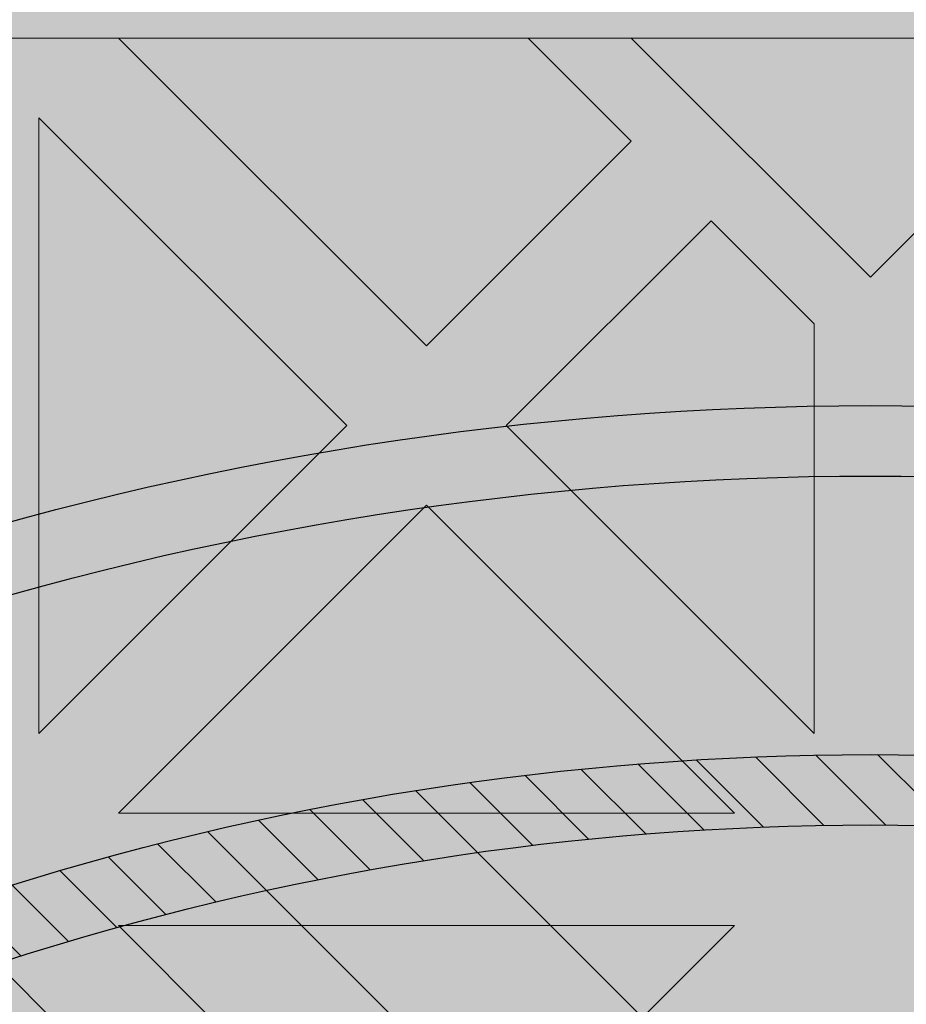
# Model space of a CAD drawing. Units: inches. Extents: x 844 to 2234, y 346 to 1084.
# Tile 81 of 93: x 2001.933 to 2003.94, y 708.742 to 710.971. Entities that reach past the tile are written whole.
import ezdxf

# ---------------------------------------------------------------- set-up
doc = ezdxf.new("R2010")
doc.units = ezdxf.units.IN
doc.header["$MEASUREMENT"] = 0
for name, color, linetype, lineweight in [('A-ANNO-DIMS', 2, 'Continuous', 18), ('furniture', 8, 'Continuous', 18), ('RA-AP-01$0$INT', 35, 'Continuous', 5)]:
    doc.layers.add(name, color=color, linetype=linetype, lineweight=lineweight)
doc.layers.add('RA-AP-01$0$FURN', color=3, linetype='Continuous')
doc.layers.add('RA-AP-01$0$WOOD', color=64, linetype='Continuous')
doc.styles.get("Standard").update_dxf_attribs({"font": 'arial.ttf'})
doc.dimstyles.get("Standard").update_dxf_attribs({"dimtxt": 6, "dimasz": 3, "dimexe": 0.18, "dimexo": 0.0625, "dimgap": 0.09, "dimtad": 0, "dimtih": 1, "dimtoh": 1, "dimdec": 1, "dimzin": 0, "dimdsep": 46, "dimlunit": 3, "dimtxsty": 'Standard', "dimblk": 'ARCHTICK', "dimcen": 0.09, "dimadec": 0, "dimazin": 0, "dimtfac": 1, "dimtdec": 1, "dimtofl": 0, "dimtmove": 0, "dimatfit": 3, "dimfxl": 1, "dimtolj": 1, "dimtzin": 0, "dimarcsym": 0})

# ---------------------------------------------------------------- blocks, each defined once
blk = doc.blocks.new('A$C18D01794')
at = {"layer": 'RA-AP-01$0$INT'}
blk.add_hatch(color=256, dxfattribs=at).paths.add_polyline_path([(4.505206456958071, -7.906712009588039), (5.305206456958072, -7.906712009588039), (5.305206456958072, -7.106712009588038), (5.255206456951893, -7.106712009588036), (5.25520645694868, -7.856712009570104), (4.555206456959269, -7.856712009588616), (4.555206456956052, -7.106712009588038), (4.505206456958073, -7.106712009588038)])
h = blk.add_hatch(color=256, dxfattribs=at)
h.paths.add_polyline_path([(4.585917135068448, -7.856712009587804), (4.614201406330596, -7.856712009587056), (4.668846067270487, -7.802067348644738), (4.723490728212344, -7.856712009584164), (4.771774999457151, -7.856712009582887), (4.826419660396886, -7.80206734864072), (4.862780050090322, -7.838427738332541), (4.844495778842715, -7.856712009580965), (4.862780050090411, -7.856712009580482), (4.905206456960182, -7.814285602707865), (4.947632863832445, -7.856712009578238), (4.965917135079675, -7.856712009577755), (4.947632863831759, -7.838427738330656), (4.983993253523576, -7.802067348637219), (5.038637914464627, -7.856712009575829), (5.08692218571208, -7.856712009574554), (5.141566846649976, -7.802067348634224), (5.196211507589851, -7.856712009571666), (5.224495778822615, -7.856712009570916), (4.905206456953975, -7.537422687702283)])
h.paths.add_polyline_path([(4.895206456956031, -7.575706958950402), (4.895206456958921, -7.684996280828174), (4.840561796018589, -7.630351619890275)], flags=16)
h.paths.add_polyline_path([(4.915206456955638, -7.575706958949956), (4.969851117895509, -7.630351619887399), (4.915206456957609, -7.684996280827732)], flags=16)
h.paths.add_polyline_path([(4.826419660395175, -7.644493755514321), (4.881064321335613, -7.699138416452331), (4.771774999456703, -7.69913841645522)], flags=16)
h.paths.add_polyline_path([(4.983993253519558, -7.644493755510815), (5.038637914460456, -7.699138416449285), (4.929348592581548, -7.69913841645126)], flags=16)
h.paths.add_polyline_path([(4.881064321336025, -7.719138416452334), (4.826419660397532, -7.773783077393256), (4.771774999457062, -7.719138416455217)], flags=16)
h.paths.add_polyline_path([(4.929348592582019, -7.71913841645126), (5.038637914460982, -7.719138416449284), (4.983993253522945, -7.773783077389749)], flags=16)
h.paths.add_polyline_path([(4.895206456960191, -7.733280552075633), (4.895206456962115, -7.806001331460164), (4.876922185715016, -7.824285602708492), (4.840561796021581, -7.787925213016675)], flags=16)
h.paths.add_polyline_path([(4.915206456958487, -7.733280552075187), (4.969851117899527, -7.787925213013798), (4.933490728206909, -7.824285602708034), (4.9152064569598, -7.806001331461736)], flags=16)
h.paths.add_polyline_path([(4.757632863832376, -7.733280552079264), (4.812277524772842, -7.787925213017304), (4.757632863834348, -7.842569873958233)], flags=16)
h.paths.add_polyline_path([(4.737632863832376, -7.73328055207979), (4.737632863834348, -7.842569873958701), (4.682988202893906, -7.787925213020692)], flags=16)
h.paths.add_polyline_path([(5.05278005008503, -7.733280552072701), (5.052780050087917, -7.842569873951664), (4.998135389146995, -7.787925213013169)], flags=16)
h.paths.add_polyline_path([(5.072780050085024, -7.733280552072333), (5.127424711025931, -7.787925213010806), (5.072780050087916, -7.842569873951244)], flags=16)
h.paths.add_polyline_path([(4.935917135072783, -7.506712009583784), (5.255206456948811, -7.826001331459767), (5.255206456948932, -7.797717060211899), (5.200561796010279, -7.743072399273238), (5.255206456949403, -7.688427738334128), (5.25520645694961, -7.640143467086677), (5.200561796009787, -7.585498806146837), (5.236922185702417, -7.549138416454212), (5.255206456949919, -7.56742268770172), (5.255206456949998, -7.549138416454178), (5.212780050078687, -7.506712009583814), (5.25520645695036, -7.464285602712145), (5.255206456950438, -7.446001331464763), (5.236922185702424, -7.464285602712779), (5.200561796009796, -7.427925213020149), (5.255206456950753, -7.373280552079203), (5.25520645695096, -7.324996280834394), (5.200561796010322, -7.270351619893748), (5.255206456951428, -7.215706958952649), (5.255206456951547, -7.187422687705071)])
h.paths.add_polyline_path([(5.042988202883395, -7.42792521302065), (5.097632863823085, -7.373280552080975), (5.097632863822622, -7.482569873959883)], flags=16)
h.paths.add_polyline_path([(5.028846067259663, -7.442067348644384), (5.083490728198774, -7.496712009583504), (4.974201406321001, -7.496712009583035)], flags=16)
h.paths.add_polyline_path([(5.117632863823087, -7.37328055208089), (5.172277524762331, -7.42792521302015), (5.11763286382262, -7.482569873959851)], flags=16)
h.paths.add_polyline_path([(5.08349072819877, -7.516712009582191), (5.028846067259652, -7.571356670521302), (4.974201406320998, -7.516712009582638)], flags=16)
h.paths.add_polyline_path([(5.131774999446817, -7.35913841645716), (5.186419660386065, -7.413783077396415), (5.241064321325782, -7.359138416456712)], flags=17)
h.paths.add_polyline_path([(5.131774999446228, -7.496712009583703), (5.186419660386065, -7.442067348643883), (5.222780050079488, -7.478427738337313), (5.204495778832781, -7.496712009584014)], flags=16)
h.paths.add_polyline_path([(5.097632863822613, -7.530854145205813), (5.097632863823061, -7.640143467084723), (5.042988202883383, -7.585498806145032)], flags=16)
h.paths.add_polyline_path([(5.131774999446899, -7.339138416457162), (5.241064321325809, -7.339138416456712), (5.186419660386591, -7.284493755517479)], flags=17)
h.paths.add_polyline_path([(5.131774999446226, -7.516712009581999), (5.204495778830767, -7.516712009581702), (5.22278005007868, -7.534996280829206), (5.186419660386049, -7.571356670521828)], flags=16)
h.paths.add_polyline_path([(5.11763286382262, -7.530854145205852), (5.17227752476232, -7.585498806145562), (5.117632863823064, -7.64014346708481)], flags=16)
h.paths.add_polyline_path([(5.186419660386069, -7.599640941770585), (5.241064321325754, -7.654285602710281), (5.131774999446791, -7.654285602709814)], flags=16)
h.paths.add_polyline_path([(5.131774999446872, -7.674285602709813), (5.24106432132578, -7.674285602710282), (5.186419660386554, -7.728930263649504)], flags=16)
h.paths.add_polyline_path([(5.255206456951811, -7.126001331467467), (5.255206456951895, -7.106712009588038), (4.555206456956052, -7.106712009588038), (4.555206456956136, -7.12600133146746), (4.905206456953973, -7.476001331465289)])
h.paths.add_polyline_path([(4.983993253513404, -7.368930263651977), (4.92934859257295, -7.314285602713969), (5.03863791445186, -7.314285602711063)], flags=16)
h.paths.add_polyline_path([(4.969851117889988, -7.383072399276016), (4.915206456952556, -7.437717060215906), (4.915206456949648, -7.328427738338133)], flags=16)
h.paths.add_polyline_path([(4.929348592572535, -7.294285602713971), (4.983993253511019, -7.239640941773039), (5.038637914451496, -7.294285602711065)], flags=16)
h.paths.add_polyline_path([(5.052780050074912, -7.280143467087016), (4.998135389134438, -7.225498806148989), (5.052780050072919, -7.170854145208052)], flags=16)
h.paths.add_polyline_path([(5.07278005007491, -7.280143467086489), (5.072780050072918, -7.170854145207579), (5.127424711013374, -7.225498806145578)], flags=16)
h.paths.add_polyline_path([(4.89520645695295, -7.437717060216355), (4.840561796013067, -7.383072399278919), (4.895206456950961, -7.328427738338582)], flags=16)
h.paths.add_polyline_path([(4.915206456948365, -7.280143467090674), (4.915206456946434, -7.207422687704125), (4.933490728192729, -7.18913841645701), (4.969851117886972, -7.225498806149623)], flags=16)
h.paths.add_polyline_path([(4.881064321327021, -7.314285602715054), (4.82641966038902, -7.368930263655506), (4.771774999448108, -7.314285602717047)], flags=16)
h.paths.add_polyline_path([(4.895206456950073, -7.280143467091125), (4.840561796009022, -7.225498806152518), (4.876922185700835, -7.18913841645908), (4.895206456948749, -7.207422687706589)], flags=16)
h.paths.add_polyline_path([(4.983993253510392, -7.211356670525576), (4.947632863816944, -7.174996280833758), (4.965917135064043, -7.156712009585847), (5.038637914448995, -7.156712009584522)], flags=16)
h.paths.add_polyline_path([(4.881064321326543, -7.294285602715056), (4.771774999447578, -7.294285602717046), (4.826419660385607, -7.239640941776569)], flags=16)
h.paths.add_polyline_path([(4.905206456946447, -7.19913841645844), (4.862780050074785, -7.156712009587725), (4.947632863816685, -7.156712009586302)], flags=16)
h.paths.add_polyline_path([(5.14156684663679, -7.211356670521528), (5.086922185696452, -7.156712009583639), (5.196211507574223, -7.156712009581651)], flags=16)
h.paths.add_polyline_path([(4.8264196603837, -7.211356670529104), (4.771774999442643, -7.156712009590501), (4.8444957788276, -7.156712009588568), (4.862780050075511, -7.17499628083566)], flags=16)
h.paths.add_polyline_path([(4.812277524760289, -7.225498806153156), (4.757632863822258, -7.28014346709363), (4.757632863819352, -7.170854145214669)], flags=16)
h.paths.add_polyline_path([(4.73763286382226, -7.280143467093997), (4.682988202881349, -7.22549880615554), (4.737632863819352, -7.170854145215086)], flags=16)
h.paths.add_polyline_path([(4.723490728195188, -7.156712009591787), (4.668846067257299, -7.211356670532127), (4.614201406317417, -7.156712009594693)], flags=16)
h.paths.add_polyline_path([(4.597632863829262, -7.506712009583814), (4.555206456957951, -7.54913841645418), (4.555206456958029, -7.56742268770172), (4.573490728205535, -7.549138416454212), (4.609851117898167, -7.585498806146839), (4.555206456958338, -7.640143467086675), (4.555206456958546, -7.688427738334125), (4.60985111789767, -7.743072399273238), (4.555206456959015, -7.797717060211899), (4.555206456959138, -7.826001331459767), (4.874495778835167, -7.506712009583786), (4.5552064569564, -7.187422687705062), (4.555206456956523, -7.215706958952644), (4.609851117897629, -7.270351619893746), (4.555206456956988, -7.324996280834396), (4.555206456957198, -7.373280552079195), (4.609851117898153, -7.427925213020147), (4.573490728205528, -7.464285602712779), (4.555206456957507, -7.446001331464756), (4.555206456957585, -7.464285602712143)])
h.paths.add_polyline_path([(4.712780050085332, -7.482569873959882), (4.712780050084863, -7.373280552080972), (4.767424711024555, -7.42792521302065)], flags=16)
h.paths.add_polyline_path([(4.726922185709173, -7.496712009583504), (4.781566846648288, -7.442067348644384), (4.836211507586949, -7.496712009583033)], flags=16)
h.paths.add_polyline_path([(4.692780050085327, -7.482569873959851), (4.638135389145619, -7.427925213020149), (4.692780050084865, -7.373280552080892)], flags=16)
h.paths.add_polyline_path([(4.726922185709182, -7.516712009582191), (4.836211507586949, -7.51671200958264), (4.7815668466483, -7.571356670521304)], flags=16)
h.paths.add_polyline_path([(4.678637914461726, -7.496712009583706), (4.605917135075169, -7.496712009584014), (4.587632863828464, -7.478427738337311), (4.623993253521887, -7.442067348643881)], flags=16)
h.paths.add_polyline_path([(4.712780050085336, -7.530854145205816), (4.767424711024568, -7.585498806145034), (4.71278005008489, -7.640143467084724)], flags=16)
h.paths.add_polyline_path([(4.678637914461726, -7.516712009582001), (4.623993253521899, -7.571356670521829), (4.587632863829271, -7.534996280829206), (4.605917135077185, -7.5167120095817)], flags=16)
h.paths.add_polyline_path([(4.692780050085336, -7.530854145205848), (4.692780050084889, -7.64014346708481), (4.638135389145632, -7.585498806145562)], flags=16)
h.paths.add_polyline_path([(4.623993253521885, -7.413783077396415), (4.678637914461131, -7.359138416457161), (4.56934859258217, -7.359138416456712)], flags=17)
h.paths.add_polyline_path([(4.623993253521901, -7.599640941770568), (4.678637914461158, -7.654285602709814), (4.569348592582195, -7.654285602710281)], flags=16)
h.paths.add_polyline_path([(4.678637914461051, -7.339138416457162), (4.623993253521361, -7.284493755517479), (4.569348592582143, -7.339138416456712)], flags=17)
h.paths.add_polyline_path([(4.678637914461076, -7.674285602709813), (4.623993253521399, -7.728930263649504), (4.569348592582167, -7.674285602710281)], flags=16)
h = blk.add_hatch(color=256, dxfattribs=at)
h.paths.add_polyline_path([(4.905206456954232, -7.537422687702028), (4.874495778835232, -7.506712009583718), (4.555206456959138, -7.826001331459766), (4.555206456959269, -7.856712009588616), (4.585917135068449, -7.856712009587804)])
h.paths.add_polyline_path([(4.935917135072152, -7.506712009583152), (4.905206456953497, -7.537422687701806), (5.224495778822614, -7.856712009570917), (5.255206456948681, -7.856712009570104), (5.255206456948813, -7.826001331459768)])
h.paths.add_polyline_path([(5.255206456951549, -7.18742268770507), (5.255206456951813, -7.126001331467461), (4.905206456953563, -7.476001331465701), (4.935917135072559, -7.506712009584006)])
h.paths.add_polyline_path([(4.874495778835167, -7.506712009583785), (4.905206456953818, -7.476001331465132), (4.555206456956135, -7.126001331467458), (4.555206456956399, -7.187422687705064)])
h = blk.add_hatch(color=256, dxfattribs=at)
h.paths.add_polyline_path([(4.969851117891331, -7.630351619889621), (4.915206456952669, -7.575706958950966), (4.915206456952222, -7.684996280828739)])
h.paths.add_polyline_path([(4.895206456953064, -7.575706958950968), (4.840561796014413, -7.630351619889628), (4.895206456953533, -7.684996280828741)])
h.paths.add_polyline_path([(4.826419660390684, -7.644493755513362), (4.771774999451003, -7.699138416453052), (4.881064321329913, -7.699138416452587)])
h.paths.add_polyline_path([(4.881064321329884, -7.719138416452585), (4.771774999450921, -7.719138416453052), (4.82641966039018, -7.773783077392298)])
h.paths.add_polyline_path([(4.895206456953734, -7.733280552076196), (4.840561796013912, -7.787925213016031), (4.876922185707337, -7.824285602709455), (4.895206456954043, -7.806001331462747)])
h.paths.add_polyline_path([(4.862780050082808, -7.838427738332388), (4.826419660390178, -7.802067348639763), (4.771774999450351, -7.856712009579595), (4.844495778835303, -7.856712009579895)])
h.paths.add_polyline_path([(4.812277524766446, -7.787925213016036), (4.757632863827191, -7.733280552076788), (4.757632863826741, -7.842569873955747)])
h.paths.add_polyline_path([(4.737632863827191, -7.733280552076863), (4.682988202887508, -7.787925213016558), (4.737632863826743, -7.842569873955778)])
h.paths.add_polyline_path([(4.668846067263777, -7.802067348640287), (4.614201406325123, -7.856712009578949), (4.723490728202894, -7.856712009579402)])
h.paths.add_polyline_path([(4.905206456953846, -7.814285602708654), (4.862780050082654, -7.856712009579847), (4.947632863824561, -7.85671200958032)])
h.paths.add_polyline_path([(4.915206456952028, -7.733280552076195), (4.91520645695173, -7.806001331460731), (4.933490728199234, -7.824285602708648), (4.96985111789186, -7.787925213016022)])
h.paths.add_polyline_path([(5.038637914454841, -7.719138416453029), (4.929348592575874, -7.71913841645258), (4.983993253515593, -7.773783077392289)])
h.paths.add_polyline_path([(4.983993253515065, -7.644493755513352), (4.929348592575849, -7.699138416452582), (5.038637914454755, -7.699138416453031)])
h.paths.add_polyline_path([(5.052780050079843, -7.73328055207676), (4.998135389140595, -7.787925213016018), (5.052780050080309, -7.842569873955721)])
h.paths.add_polyline_path([(4.983993253516868, -7.802067348639752), (4.947632863824241, -7.838427738332383), (4.965917135071747, -7.856712009579888), (5.038637914456701, -7.856712009579572)])
h.paths.add_polyline_path([(5.127424711019533, -7.787925213016519), (5.072780050079843, -7.733280552076838), (5.07278005008031, -7.842569873955751)])
h.paths.add_polyline_path([(5.141566846643269, -7.802067348640248), (5.086922185704154, -7.85671200957937), (5.196211507581929, -7.856712009578901)])
for p, q in [((4.905206456953975, -7.537422687702283), (5.224495778822613, -7.856712009570916)), ((4.929348592581546, -7.69913841645126), (4.983993253519556, -7.644493755510815)), ((4.983993253519558, -7.644493755510817), (5.038637914460456, -7.699138416449285)), ((5.038637914460456, -7.699138416449285), (4.929348592581546, -7.69913841645126)), ((5.038637914460983, -7.719138416449284), (4.92934859258202, -7.71913841645126)), ((4.92934859258202, -7.71913841645126), (4.983993253522945, -7.773783077389751)), ((5.038637914460983, -7.719138416449284), (4.983993253522945, -7.773783077389751)), ((4.9152064569598, -7.806001331460137), (4.915206456958485, -7.733280552075186)), ((4.915206456958485, -7.733280552075186), (4.969851117899529, -7.787925213013799)), ((5.052780050085028, -7.733280552072701), (4.998135389146995, -7.787925213013169)), ((5.052780050085028, -7.733280552072701), (5.052780050087917, -7.842569873951664)), ((4.969851117899529, -7.787925213013798), (4.93349072820771, -7.824285602707234)), ((5.052780050087917, -7.842569873951664), (4.998135389146995, -7.787925213013169)), ((4.983993253523578, -7.802067348637216), (4.947632863831757, -7.838427738330654)), ((5.038637914464623, -7.856712009575828), (4.983993253523576, -7.802067348637216)), ((4.915206456959793, -7.806001331461731), (4.933490728207705, -7.82428560270883)), ((4.905206456960184, -7.814285602707865), (4.862780050090411, -7.856712009580478)), ((4.905206456960184, -7.814285602707865), (4.947632863832319, -7.856712009578112)), ((4.947632863831757, -7.838427738330654), (4.965917135079625, -7.856712009577703)), ((4.965917135079672, -7.856712009577751), (4.947632863831755, -7.838427738330654)), ((4.555206456959269, -7.856712009588616), (5.255206456948681, -7.856712009570104)), ((4.947632863832319, -7.856712009578112), (4.862780050090411, -7.856712009580478)), ((4.965917135079672, -7.85671200957775), (5.038637914464623, -7.856712009575828))]:
    blk.add_line(p, q, dxfattribs=at)
blk = doc.blocks.new('A$C32926AE1')
at = {"layer": 'RA-AP-01$0$WOOD'}
h = blk.add_hatch(color=256, dxfattribs=at)
h.dxf.hatch_style = 1
h.paths.add_polyline_path([(5.157430609644524, 4.573483066760929, -0.1009492694046607), (5.155401577623758, 4.593365984175333, -0.1842662638101597), (5.172249623284174, 4.638795604568598, 0.2056608120311276), (5.179560981299304, 4.661316324430096, 0.3614336704623542), (5.134352340494423, 4.706524965234944, 0.2056608120311297), (5.111831620632933, 4.699213607219793, -0.1842662638101113), (5.066402000239693, 4.682365561559342, -0.1055311479399994), (5.045656153913092, 4.68467289944697, 0.1567636581983829), (4.763886414745334, 4.684672899446966, -0.1055311479399895), (4.743140568418733, 4.68236556155934, -0.1842662638100833), (4.6977109480255, 4.69921360721979, 0.2056608120302612), (4.675190228164109, 4.706524965234949, 0.3614336704708441), (4.629981587358889, 4.66131632442871, 0.2056608120245944), (4.637292945374126, 4.638795604567974, -0.1842662638101024), (4.654140991034615, 4.59336598417475, -0.1009492694055169), (4.652111959013835, 4.573483066760181, 0.021410119221476), (4.629748025606143, 4.156712009541676, 0.0214101192214795), (4.652111959013809, 3.739940952323101, -0.1009492694059586), (4.654140991034615, 3.720058034908448, -0.1842662638100975), (4.637292945374126, 3.674628414515226, 0.2056608120245705), (4.629981587358889, 3.652107694654492, 0.3614336704708879), (4.675190228164113, 3.606899053848249, 0.2056608120302384), (4.697710948025501, 3.614210411863408, -0.1842662638100995), (4.743140568418738, 3.63105845752386, -0.1055311479402541), (4.763886414745388, 3.628751119636215, 0.1567636581983776), (5.045656153913137, 3.628751119636244, -0.1055311479397538), (5.066402000239692, 3.631058457523857, -0.1842662638101067), (5.111831620632931, 3.614210411863407, 0.2056608120310924), (5.134352340494417, 3.606899053848256, 0.3614336704624001), (5.179560981299307, 3.652107694653103, 0.2056608120311314), (5.172249623284175, 3.6746284145146, -0.1842662638101402), (5.155401577623758, 3.72005803490786, -0.1009492694051366), (5.15743060964455, 3.739940952322354, 0.0214101192215073), (5.179794543052287, 4.156712009541468, 0.0214101192215252)])
h.paths.add_polyline_path([(4.639748609479751, 4.156712009541513, 0.0213537860821624), (4.661970494867118, 3.741887061152232, -0.094075836301374), (4.664143710413708, 3.7196126951003, -0.1824818158568985), (4.644813765429836, 3.668037719127816, 0.2056608120245319), (4.639939526753007, 3.653023905887301, 0.3614336704710246), (4.676106439397173, 3.616856993242342, 0.2056608120302234), (4.691120252638095, 3.621731231919122, -0.1824818158602558), (4.742695228611606, 3.641061176902986, -0.1029891339458722), (4.766991894714349, 3.638256818950944, 0.156709409989566), (5.042550673941472, 3.638256818950105, -0.102989133958497), (5.066847340047078, 3.641061176902949, -0.1824818158594995), (5.118422316020358, 3.621731231919103, 0.2056608120311416), (5.133436129261316, 3.616856993242346, 0.3614336704621468), (5.169603041905217, 3.653023905886178, 0.2056608120310986), (5.164728803228477, 3.668037719127177, -0.1824818158565612), (5.145398858244737, 3.719612695099578, -0.0940758363009313), (5.147572073791232, 3.741887061151398, 0.0213537860822023), (5.169793959178681, 4.156712009541451, 0.0213537860822226), (5.147572073791203, 4.571536957931898, -0.0940758363005034), (5.145398858244737, 4.59381132398362, -0.1824818158565587), (5.164728803228476, 4.645386299956021, 0.2056608120311045), (5.169603041905216, 4.66040011319702, 0.3614336704621845), (5.133436129261313, 4.696567025840856, 0.2056608120310773), (5.118422316020359, 4.691692787164098, -0.182481815859508), (5.066847340047078, 4.67236284218025, -0.1029891339584606), (5.04255067394148, 4.675167200133092, 0.156709409989566), (4.766991894714357, 4.675167200132257, -0.1029891339458842), (4.742695228611611, 4.672362842180213, -0.1824818158602725), (4.691120252638095, 4.691692787164077, 0.2056608120302152), (4.676106439397174, 4.696567025840858, 0.3614336704710363), (4.639939526753005, 4.660400113195899, 0.2056608120245495), (4.644813765429837, 4.645386299955384, -0.1824818158568934), (4.664143710413708, 4.593811323982902, -0.0940758363009187), (4.661970494867149, 4.571536957931074, 0.021353786082177)], flags=16)
h.paths.add_polyline_path([(5.129794543052235, 4.432167055276933, -0.0141661062790638), (5.130152669293814, 4.156927903047693, -0.0141661062790647), (5.129794543052234, 3.881688750818433, -0.0785247771143638), (5.10979738006795, 3.755143611847103, 0.0945969212073497), (5.105408519571111, 3.717898134952927, 0.1043170707844957), (5.116074640131521, 3.670385395016088, 0.1043170707864965), (5.068561900193738, 3.681051515576561, 0.09459692119553), (5.031316423304057, 3.676662655080835, -0.1580239521427272), (4.778226145355827, 3.676662655080367, 0.0945969211986668), (4.740980668464973, 3.681051515576592, 0.1043170707882822), (4.693467928526415, 3.670385395015844, 0.1043170707867916), (4.704134049087309, 3.717898134953662, 0.0945969211972894), (4.69974518859162, 3.755143611844042, -0.0785247771163196), (4.679748025606343, 3.881688750818406, -0.0141661062790663), (4.679389899364763, 4.156927903047693, -0.0141661062790672), (4.679748025606343, 4.432167055276998, -0.0785247771163064), (4.699745188591625, 4.55871219425134, 0.094596921197333), (4.704134049087308, 4.595957671141738, 0.1043170707867205), (4.693467928526416, 4.643470411079523, 0.1043170707882628), (4.740980668464965, 4.632804290518776, 0.0945969211988114), (4.778226145355874, 4.637193151015016, -0.158023952142669), (5.031316423304015, 4.637193151014546, 0.0945969211956361), (5.068561900193736, 4.632804290518806, 0.1043170707864979), (5.11607464013152, 4.643470411079278, 0.1043170707844617), (5.105408519571112, 4.595957671142455, 0.0945969212074597), (5.109797380067959, 4.558712194248236, -0.0785247771143467)], flags=0)
h.paths.add_polyline_path([(5.119794532311105, 4.432259799204851, -0.0142000800617244), (5.120156169157484, 4.156927903047701, -0.0142000800617277), (5.119794532311105, 3.881596006890482, -0.0784894509520253), (5.100273383573699, 3.758192358677797, 0.0940138827242913), (5.095413455884425, 3.717477693979438, 0.0606271852308753), (5.099615656341024, 3.686844378806616, 0.0606271852322524), (5.068982341167493, 3.691046579263239, 0.0940138827010453), (5.028267676478798, 3.686186651576848, -0.1580706864508061), (4.781274892180912, 3.686186651576435, 0.0940138827026903), (4.740560227491556, 3.691046579263279, 0.0606271852339895), (4.709926912317155, 3.686844378806508, 0.0606271852329405), (4.714129112773991, 3.717477693980356, 0.094013882701304), (4.709269185087677, 3.758192358669163, -0.0784894509577193), (4.689748036347473, 3.881596006890469, -0.014200080061729), (4.689386399501094, 4.156927903047709, -0.0142000800617217), (4.689748036347473, 4.432259799204808, -0.078489450957724), (4.709269185087651, 4.555663447426125, 0.0940138827014585), (4.714129112773992, 4.596378112114996, 0.0606271852329731), (4.709926912317154, 4.62701142728886, 0.0606271852340196), (4.74056022749157, 4.622809226832087, 0.0940138827024997), (4.781274892180847, 4.627669154518912, -0.1580706864508359), (5.028267676478777, 4.627669154518526, 0.0940138827010946), (5.068982341167492, 4.622809226832129, 0.060627185232254), (5.099615656341024, 4.627011427288751, 0.0606271852308727), (5.095413455884425, 4.59637811211593, 0.0940138827241088), (5.100273383573675, 4.555663447417647, -0.0784894509520978)], flags=0)
h.paths.add_polyline_path([(5.06978912287499, 4.430218106756144, -0.014241683694547), (5.070173729147532, 4.156927903047672, -0.0142416836945458), (5.06978912287499, 3.883637699339223, -0.0800609523125196), (5.052662118612511, 3.773463122773442, 0.0526421978001116), (5.04590916754064, 3.740550867606997, 0.0526421977992423), (5.012996912374707, 3.73379791653534, -0.1583028414718258), (4.796545656286308, 3.73379791653451, 0.0526421978034211), (4.763633401117837, 3.740550867607021, 0.0526421978018622), (4.756880450045755, 3.773463122774558, -0.0800609523117106), (4.739753445783639, 3.883637699339268, -0.0142416836945435), (4.739368839511098, 4.156927903047671, -0.0142416836945477), (4.739753445783639, 4.430218106756155, -0.0800609523116345), (4.75688045004574, 4.540392683320762, 0.052642197801941), (4.763633401117837, 4.573304938488346, 0.0526421978035071), (4.796545656286361, 4.580057889560873, -0.1583028414717561), (5.012996912374669, 4.580057889560039, 0.0526421977993048), (5.04590916754064, 4.57330493848837, 0.0526421978002057), (5.052662118612529, 4.540392683321868, -0.080060952312477)], flags=0)
h.paths.add_polyline_path([(5.049789715110557, 4.43038092723357, -0.0143097550741839), (5.05018085590259, 4.156927903047715, -0.0143097550741854), (5.049789715110558, 3.883474878861827, -0.0800685599149176), (5.03362098255317, 3.779581877367999, 0.0306258898956367), (5.028241146483733, 3.758218888663947, 0.0306258898977031), (5.006878157778253, 3.75283905259408, -0.1583983521624096), (4.802664410878162, 3.752839052594731, 0.0306258898946014), (4.781301422174808, 3.758218888663924, 0.0306258898967912), (4.775921586105202, 3.779581877368794, -0.080068559914251), (4.759752853548071, 3.883474878861786, -0.0143097550741854), (4.759361712756037, 4.156927903047671, -0.0143097550741854), (4.759752853548071, 4.430380927233557, -0.0800685599142479), (4.775921586105193, 4.534273928726546, 0.0306258898968306), (4.781301422174808, 4.555636917431444, 0.0306258898945754), (4.802664410878143, 4.561016753500631, -0.1583983521624168), (5.006878157778244, 4.561016753501291, 0.0306258898977177), (5.028241146483733, 4.555636917431421, 0.0306258898958182), (5.03362098255321, 4.534273928727244, -0.080068559914796)], flags=0)
h.paths.add_polyline_path([(4.999766070382627, 4.428171244713864, -0.0143443147609634), (5.000198441819402, 4.156927903047689, -0.0143443147609612), (4.999766070382627, 3.885684561381556, -0.0784641635803329), (4.987356730658798, 3.799103304488872, -0.1506053783831347), (4.822185837999821, 3.79910330448882, -0.0784641635803318), (4.809776498276007, 3.885684561381509, -0.014344314760963), (4.809344126839227, 4.156927903047677, -0.0143443147609645), (4.809776498276007, 4.428171244713873, -0.0784641635803192), (4.822185837999822, 4.514752501606549, -0.1506053783831338), (4.987356730658798, 4.514752501606494, -0.078464163580285)], flags=0)
h.paths.add_polyline_path([(4.979755254238824, 4.42764379880488, -0.0143772539198268), (4.980205517789977, 4.156927903047693, -0.0143772539198275), (4.979755254238824, 3.886212007290489, -0.0689242507424422), (4.971183264704897, 3.815276770442801, -0.1296645318904179), (4.838359303953726, 3.815276770442746, -0.0689242507424186), (4.829787314419809, 3.886212007290419, -0.0143772539198292), (4.829337050868653, 4.156927903047653, -0.0143772539198325), (4.829787314419809, 4.427643798804946, -0.0689242507424211), (4.838359303953725, 4.498579035652621, -0.1296645318904187), (4.971183264704897, 4.498579035652565, -0.0689242507424401)], flags=0)
h = blk.add_hatch(color=256, dxfattribs=at)
h.dxf.hatch_style = 1
h.paths.add_polyline_path([(5.145398858244737, 4.59381132398362, -0.1824818158565616), (5.164728803228476, 4.645386299956021, 0.2056608120311045), (5.169603041905216, 4.66040011319702, 0.3614336704621845), (5.133436129261313, 4.696567025840856, 0.2056608120310773), (5.118422316020359, 4.691692787164098, -0.182481815859508), (5.066847340047078, 4.67236284218025, -0.1029891339584606), (5.04255067394148, 4.675167200133092, 0.156709409989566), (4.766991894714357, 4.675167200132257, -0.1029891339458842), (4.742695228611611, 4.672362842180213, -0.1824818158602725), (4.691120252638095, 4.691692787164077, 0.2056608120302152), (4.676106439397174, 4.696567025840858, 0.3614336704710363), (4.639939526753005, 4.660400113195899, 0.2056608120245495), (4.644813765429837, 4.645386299955384, -0.1824818158568934), (4.664143710413708, 4.593811323982902, -0.0940758363009187), (4.661970494867149, 4.571536957931074, 0.0213537860821772), (4.639748609479751, 4.156712009541507, 0.0213537860821625), (4.661970494867119, 3.741887061152226, -0.0940758363013071), (4.664143710413708, 3.719612695100309, -0.1824818158569294), (4.644813765429836, 3.668037719127816, 0.2056608120245319), (4.639939526753007, 3.653023905887301, 0.3614336704710246), (4.676106439397173, 3.616856993242342, 0.2056608120302234), (4.691120252638095, 3.621731231919122, -0.1824818158602558), (4.742695228611606, 3.641061176902986, -0.1029891339458722), (4.766991894714349, 3.638256818950944, 0.156709409989566), (5.042550673941472, 3.638256818950105, -0.102989133958497), (5.066847340047078, 3.641061176902949, -0.1824818158594995), (5.118422316020358, 3.621731231919103, 0.2056608120311416), (5.133436129261316, 3.616856993242346, 0.3614336704621468), (5.169603041905217, 3.653023905886178, 0.2056608120310986), (5.164728803228477, 3.668037719127177, -0.1824818158565612), (5.145398858244737, 3.719612695099578, -0.0940758363009313), (5.147572073791232, 3.741887061151398, 0.0213537860822023), (5.169793959178681, 4.156712009541451, 0.0213537860822226), (5.147572073791203, 4.571536957931898, -0.0940758363004996)])
h.paths.add_polyline_path([(5.109797380067958, 4.55871219424824, -0.0785247771143472), (5.129794543052234, 4.432167055276936, -0.0141661062790644), (5.130152669293814, 4.156927903047685, -0.014166106279066), (5.129794543052234, 3.881688750818401, -0.0785247771143517), (5.109797380067946, 3.755143611847092, 0.0945969212073132), (5.105408519571111, 3.717898134952929, 0.1043170707844995), (5.116074640131521, 3.670385395016088, 0.1043170707864965), (5.068561900193738, 3.681051515576561, 0.09459692119553), (5.031316423304057, 3.676662655080835, -0.1580239521427272), (4.778226145355827, 3.676662655080367, 0.0945969211986668), (4.740980668464973, 3.681051515576592, 0.1043170707882822), (4.693467928526415, 3.670385395015844, 0.1043170707867916), (4.704134049087309, 3.717898134953662, 0.0945969211972894), (4.69974518859162, 3.755143611844042, -0.0785247771163196), (4.679748025606343, 3.881688750818406, -0.0141661062790663), (4.679389899364763, 4.156927903047693, -0.0141661062790672), (4.679748025606343, 4.432167055276998, -0.0785247771163064), (4.699745188591625, 4.55871219425134, 0.094596921197333), (4.704134049087308, 4.595957671141738, 0.1043170707867205), (4.693467928526416, 4.643470411079523, 0.1043170707882628), (4.740980668464965, 4.632804290518776, 0.0945969211988114), (4.778226145355874, 4.637193151015016, -0.158023952142669), (5.031316423304015, 4.637193151014546, 0.0945969211956361), (5.068561900193736, 4.632804290518806, 0.1043170707864979), (5.11607464013152, 4.643470411079278, 0.1043170707844617), (5.105408519571112, 4.595957671142455, 0.0945969212074504)], flags=16)
h.paths.add_polyline_path([(5.100273383573655, 4.55566344741771, -0.0784894509521388), (5.119794532311105, 4.432259799204852, -0.0142000800617252), (5.120156169157484, 4.156927903047686, -0.014200080061726), (5.119794532311105, 3.881596006890502, -0.0784894509520446), (5.100273383573696, 3.758192358677786, 0.0940138827242721), (5.095413455884425, 3.717477693979436, 0.0606271852308692), (5.099615656341024, 3.686844378806616, 0.0606271852322522), (5.068982341167493, 3.691046579263239, 0.0940138827010453), (5.028267676478798, 3.686186651576848, -0.1580706864508061), (4.781274892180912, 3.686186651576435, 0.0940138827026903), (4.740560227491556, 3.691046579263279, 0.0606271852339895), (4.709926912317155, 3.686844378806508, 0.0606271852329405), (4.714129112773991, 3.717477693980356, 0.094013882701304), (4.709269185087677, 3.758192358669163, -0.0784894509577193), (4.689748036347473, 3.881596006890469, -0.014200080061729), (4.689386399501094, 4.156927903047709, -0.0142000800617217), (4.689748036347473, 4.432259799204808, -0.078489450957724), (4.709269185087651, 4.555663447426125, 0.0940138827014585), (4.714129112773992, 4.596378112114996, 0.0606271852329731), (4.709926912317154, 4.62701142728886, 0.0606271852340196), (4.74056022749157, 4.622809226832087, 0.0940138827024997), (4.781274892180847, 4.627669154518912, -0.1580706864508359), (5.028267676478777, 4.627669154518526, 0.0940138827010946), (5.068982341167492, 4.622809226832129, 0.060627185232254), (5.099615656341024, 4.627011427288751, 0.0606271852308727), (5.095413455884425, 4.59637811211593, 0.094013882723957)], flags=0)
h.paths.add_polyline_path([(5.04590916754064, 4.57330493848837, 0.0526421978002057), (5.052662118612529, 4.540392683321868, -0.0800609523124783), (5.06978912287499, 4.430218106756142, -0.0142416836945469), (5.070173729147532, 4.156927903047672, -0.0142416836945458), (5.06978912287499, 3.883637699339223, -0.0800609523125196), (5.052662118612511, 3.773463122773442, 0.0526421978001116), (5.04590916754064, 3.740550867606997, 0.0526421977992423), (5.012996912374707, 3.73379791653534, -0.1583028414718258), (4.796545656286308, 3.73379791653451, 0.0526421978034211), (4.763633401117837, 3.740550867607021, 0.0526421978018622), (4.756880450045755, 3.773463122774558, -0.0800609523117106), (4.739753445783639, 3.883637699339268, -0.0142416836945435), (4.739368839511098, 4.156927903047671, -0.0142416836945477), (4.739753445783639, 4.430218106756155, -0.0800609523116345), (4.75688045004574, 4.540392683320762, 0.052642197801941), (4.763633401117837, 4.573304938488346, 0.0526421978035071), (4.796545656286361, 4.580057889560873, -0.1583028414717561), (5.012996912374669, 4.580057889560039, 0.0526421977993048)], flags=0)
h.paths.add_polyline_path([(5.028241146483733, 4.555636917431422, 0.0306258898956949), (5.033620982553182, 4.534273928727329, -0.0800685599148649), (5.049789715110557, 4.430380927233569, -0.0143097550741839), (5.05018085590259, 4.156927903047715, -0.0143097550741854), (5.049789715110558, 3.883474878861827, -0.0800685599149176), (5.03362098255317, 3.779581877367999, 0.0306258898956367), (5.028241146483733, 3.758218888663947, 0.0306258898977031), (5.006878157778253, 3.75283905259408, -0.1583983521624096), (4.802664410878162, 3.752839052594731, 0.0306258898946014), (4.781301422174808, 3.758218888663924, 0.0306258898967912), (4.775921586105202, 3.779581877368794, -0.080068559914251), (4.759752853548071, 3.883474878861786, -0.0143097550741854), (4.759361712756037, 4.156927903047671, -0.0143097550741854), (4.759752853548071, 4.430380927233557, -0.0800685599142479), (4.775921586105193, 4.534273928726546, 0.0306258898968306), (4.781301422174808, 4.555636917431444, 0.0306258898945754), (4.802664410878143, 4.561016753500631, -0.1583983521624168), (5.006878157778244, 4.561016753501291, 0.0306258898977174)], flags=0)
h.paths.add_polyline_path([(4.987356730658798, 4.514752501606494, -0.0784641635803018), (4.999766070382627, 4.428171244713845, -0.0143443147609637), (5.000198441819402, 4.156927903047665, -0.0143443147609622), (4.999766070382628, 3.885684561381514, -0.0784641635802952), (4.987356730658797, 3.799103304488872, -0.1506053783831338), (4.822185837999821, 3.799103304488819, -0.0784641635803342), (4.809776498276007, 3.885684561381512, -0.0143443147609628), (4.809344126839227, 4.156927903047676, -0.0143443147609646), (4.809776498276007, 4.428171244713873, -0.0784641635803192), (4.822185837999822, 4.514752501606549, -0.1506053783831338)], flags=0)
h.paths.add_polyline_path([(4.971183264704897, 4.498579035652566, -0.0689242507424384), (4.979755254238824, 4.427643798804883, -0.0143772539198276), (4.980205517789977, 4.15692790304768, -0.0143772539198258), (4.979755254238823, 3.88621200729051, -0.0689242507424628), (4.971183264704897, 3.815276770442801, -0.129664531890417), (4.838359303953726, 3.815276770442746, -0.0689242507424186), (4.829787314419809, 3.886212007290419, -0.0143772539198292), (4.829337050868653, 4.156927903047653, -0.0143772539198325), (4.829787314419809, 4.427643798804946, -0.0689242507424211), (4.838359303953725, 4.498579035652621, -0.1296645318904187)], flags=0)
h = blk.add_hatch(dxfattribs=at)
h.set_pattern_fill('ANSI31', color=256, scale=0.05, style=0)
h.set_pattern_definition([(45, (0, 0), (-0.0044194173824159, 0.0044194173824159), [])])
h.paths.add_polyline_path([(5.130152669293814, 4.156927903047704, 0.0141661062790657), (5.129794543052234, 4.432167055276982, 0.0777827904001433), (5.110168979996553, 4.557559993161921, -0.0976515123401879), (5.105408519571111, 4.595957671142454, -0.1043170707844687), (5.116074640131522, 4.64347041107928), (5.099615656341024, 4.627011427288751, 0.0606271852308727), (5.095413455884425, 4.59637811211593, 0.0940138827241088), (5.100273383573675, 4.555663447417647, -0.0784894509520972), (5.119794532311105, 4.432259799204852, -0.0142000800617252), (5.120156169157484, 4.156927903047686, -0.014200080061726), (5.119794532311105, 3.881596006890502, -0.0784894509520446), (5.100273383573696, 3.758192358677786, 0.0940138827242721), (5.095413455884425, 3.717477693979436, 0.0606271852308692), (5.099615656341024, 3.686844378806616), (5.116074640131519, 3.67038539501609, -0.1043170707844594), (5.105408519571112, 3.717898134952912, -0.0976515123401594), (5.11016897999655, 3.756295812933435, 0.0777827904001654), (5.129794543052234, 3.881688750818409, 0.0141661062790665)])
h.paths.add_polyline_path([(5.030164222210597, 3.676291055149937, -0.0976515123472002), (5.068561900193739, 3.681051515576561, -0.1043170707864927), (5.116074640131521, 3.670385395016088), (5.099615656341024, 3.686844378806616, 0.0606271852322522), (5.068982341167493, 3.691046579263239, 0.0940138827010453), (5.028267676478798, 3.686186651576848, -0.1580706864508061), (4.781274892180912, 3.686186651576435, 0.0940138827026903), (4.740560227491556, 3.691046579263279, 0.0606271852339913), (4.709926912317154, 3.686844378806508), (4.693467928526416, 3.670385395015845, -0.1043170707882796), (4.740980668464973, 3.681051515576592, -0.0976515123427246), (4.779378346446416, 3.676291055150394, 0.156512506893803)])
h.paths.add_polyline_path([(4.689748036347473, 3.881596006890472, -0.014200080061729), (4.689386399501094, 4.156927903047712, -0.0142000800617195), (4.689748036347473, 4.432259799204768, -0.078489450957742), (4.709269185087648, 4.555663447426114, 0.0940138827014821), (4.714129112773992, 4.596378112114995, 0.0606271852329748), (4.709926912317154, 4.62701142728886), (4.693467928526414, 4.643470411079524, -0.1043170707867939), (4.704134049087309, 4.595957671141706, -0.09765151234893), (4.699373588660725, 4.557559993157876, 0.0777827903975372), (4.679748025606343, 4.432167055276987, 0.0141661062790675), (4.679389899364763, 4.156927903047675, 0.0141661062790641), (4.679748025606343, 3.88168875081843, 0.0777827903975637), (4.699373588660724, 3.756295812937497, -0.0976515123490278), (4.704134049087308, 3.717898134953629, -0.1043170707867196), (4.693467928526416, 3.670385395015845), (4.709926912317155, 3.686844378806508, 0.0606271852329413), (4.714129112773991, 3.717477693980357, 0.0940138827013084), (4.709269185087676, 3.758192358669166, -0.0784894509577192)])
h.paths.add_polyline_path([(4.779378346446434, 4.63756475094498, -0.0976515123427943), (4.740980668464964, 4.632804290518776, -0.1043170707882609), (4.693467928526416, 4.643470411079523), (4.709926912317154, 4.62701142728886, 0.0606271852340196), (4.74056022749157, 4.622809226832087, 0.0940138827024997), (4.781274892180847, 4.627669154518912, -0.1580706864508359), (5.028267676478777, 4.627669154518526, 0.0940138827010946), (5.068982341167492, 4.622809226832129, 0.060627185232254), (5.099615656341024, 4.627011427288751), (5.116074640131521, 4.643470411079279, -0.1043170707865022), (5.068561900193735, 4.632804290518806, -0.0976515123475899), (5.030164222210446, 4.637564750945479, 0.1565125068936924)])
h = blk.add_hatch(dxfattribs=at)
h.set_pattern_fill('ANSI32', color=256, scale=0.2, style=0)
h.set_pattern_definition([(45, (0, 0), (-0.0530330085889911, 0.0530330085889911), []), (45, (0.035355339, 0), (-0.0530330085889911, 0.0530330085889911), [])])
h.paths.add_polyline_path([(5.119794532311105, 4.432259799204823, 0.0777015974868765), (5.10065834347252, 4.554469821747928, -0.0968902511992216), (5.095413455884425, 4.596378112115931, -0.060627185230871), (5.099615656341024, 4.627011427288751, -0.060627185232254), (5.068982341167492, 4.622809226832129, -0.0968902512198245), (5.027074050790956, 4.628054114423209, 0.1564657949319105), (4.782468517866163, 4.628054114422785, -0.0968902512152247), (4.740560227491555, 4.622809226832088, -0.0606271852339878), (4.709926912317155, 4.627011427288859, -0.0606271852329413), (4.714129112773991, 4.596378112115011, -0.0968902512205338), (4.708884225182929, 4.554469821738175, 0.0777015974804443), (4.689748036347473, 4.43225979920482, 0.0142000800617215), (4.689386399501094, 4.156927903047726, 0.0142000800617273), (4.689748036347473, 3.88159600689052, 0.077701597480541), (4.708884225182985, 3.759385984357019, -0.096890251220082), (4.714129112773992, 3.717477693980371, -0.0606271852329731), (4.709926912317154, 3.686844378806507, -0.060627185233988), (4.740560227491554, 3.691046579263279, -0.0968902512152569), (4.782468517866175, 3.685801691672578, 0.1564657949319236), (5.027074050790988, 3.685801691672169, -0.0968902512197451), (5.068982341167491, 3.691046579263239, -0.0606271852322557), (5.099615656341024, 3.686844378806616, -0.0606271852308727), (5.095413455884425, 3.717477693979438, -0.0968902511991229), (5.100658343472507, 3.7593859843474, 0.0777015974868745), (5.119794532311105, 3.8815960068905, 0.014200080061726), (5.120156169157484, 4.156927903047685, 0.0142000800617238)])
h.paths.add_polyline_path([(5.070173729147531, 4.156927903047684, -0.0142416836945481), (5.06978912287499, 3.883637699339191, -0.0800609523125107), (5.052662118612505, 3.773463122773424, 0.0526421978000811), (5.04590916754064, 3.740550867606997, 0.0526421977993214), (5.012996912374658, 3.733797916535325, -0.1583028414717916), (4.796545656286304, 3.733797916534512, 0.0526421978034138), (4.763633401117837, 3.740550867607021, 0.0526421978018622), (4.756880450045755, 3.773463122774558, -0.0800609523117106), (4.739753445783639, 3.883637699339268, -0.0142416836945435), (4.739368839511098, 4.156927903047671, -0.0142416836945477), (4.739753445783639, 4.430218106756155, -0.0800609523116345), (4.75688045004574, 4.540392683320762, 0.052642197801941), (4.763633401117837, 4.573304938488346, 0.0526421978035071), (4.796545656286361, 4.580057889560873, -0.1583028414717561), (5.012996912374669, 4.580057889560039, 0.0526421977993048), (5.04590916754064, 4.57330493848837, 0.0526421978002057), (5.052662118612529, 4.540392683321868, -0.0800609523124783), (5.06978912287499, 4.430218106756142, -0.0142416836945463)], flags=16)
h.paths.add_polyline_path([(5.050180855902591, 4.156927903047686, -0.0143097550741856), (5.049789715110558, 3.883474878861795, -0.0800685599148126), (5.033620982553202, 3.7795818773681, 0.0306258898957837), (5.028241146483733, 3.758218888663947, 0.0306258898977031), (5.006878157778253, 3.75283905259408, -0.1583983521624096), (4.802664410878162, 3.752839052594731, 0.0306258898946014), (4.781301422174808, 3.758218888663924, 0.0306258898967912), (4.775921586105202, 3.779581877368794, -0.080068559914251), (4.759752853548071, 3.883474878861786, -0.0143097550741854), (4.759361712756037, 4.156927903047671, -0.0143097550741854), (4.759752853548071, 4.430380927233557, -0.0800685599142479), (4.775921586105193, 4.534273928726546, 0.0306258898968306), (4.781301422174808, 4.555636917431444, 0.0306258898945754), (4.802664410878143, 4.561016753500631, -0.1583983521624168), (5.006878157778244, 4.561016753501291, 0.0306258898977177), (5.028241146483733, 4.555636917431421, 0.0306258898958182), (5.03362098255321, 4.534273928727244, -0.0800685599147973), (5.049789715110557, 4.430380927233568, -0.0143097550741854)], flags=0)
h.paths.add_polyline_path([(5.000198441819402, 4.15692790304769, -0.0143443147609622), (4.999766070382627, 3.885684561381539, -0.0784641635803169), (4.987356730658798, 3.799103304488873, -0.1506053783831347), (4.822185837999821, 3.79910330448882, -0.0784641635803318), (4.809776498276007, 3.885684561381509, -0.014344314760963), (4.809344126839227, 4.156927903047677, -0.0143443147609645), (4.809776498276007, 4.428171244713873, -0.0784641635803192), (4.822185837999822, 4.514752501606549, -0.1506053783831338), (4.987356730658798, 4.514752501606494, -0.0784641635803018), (4.999766070382627, 4.428171244713845, -0.0143443147609624)], flags=0)
h.paths.add_polyline_path([(4.980205517789976, 4.156927903047707, -0.0143772539198295), (4.979755254238824, 3.886212007290466, -0.06892425074242), (4.971183264704897, 3.815276770442801, -0.129664531890417), (4.838359303953726, 3.815276770442746, -0.0689242507424186), (4.829787314419809, 3.886212007290419, -0.0143772539198292), (4.829337050868653, 4.156927903047653, -0.0143772539198325), (4.829787314419809, 4.427643798804946, -0.0689242507424211), (4.838359303953725, 4.498579035652621, -0.1296645318904187), (4.971183264704897, 4.498579035652565, -0.0689242507424418), (4.979755254238824, 4.427643798804878, -0.0143772539198259)], flags=0)
for centre, radius, start, end in [((4.904771284329219, 4.246361343706563), 0.4603971832811766, 72.06839084771535, 107.9316091522852), ((4.904771284329217, 4.246361343706564), 0.4503971832811742, 72.06232351293878, 107.9376764867364), ((4.904771284329219, 4.246793130718732), 0.4103971832811756, 72.04030024486354, 107.9596997549356), ((4.904771284329219, 4.246793130718733), 0.4003971832811741, 72.03507539883653, 107.9649246009689)]:
    blk.add_arc(centre, radius, start, end, dxfattribs=at)
blk = doc.blocks.new('A$C5D2F253E')
at = {"layer": 'RA-AP-01$0$FURN', "xscale": -0.7999999999883585, "yscale": 0.7999999999883585, "zscale": 0.8, "rotation": 90}
blk.add_blockref('A$C18D01794', (-5.687757199772477, 4.75791982714071), dxfattribs=at)
at = {"layer": 'RA-AP-01$0$WOOD', "rotation": 270}
blk.add_blockref('A$C32926AE1', (-4.161339601644158, 5.73852594588169), dxfattribs=at)
blk = doc.blocks.new('_ArchTick')
at = {"color": 0, "linetype": 'ByBlock', "const_width": 0.15}
blk.add_lwpolyline([(-0.5, -0.5), (0.5, 0.5)], dxfattribs=at)
blk = doc.blocks.new('*D121')
at = {"layer": 'A-ANNO-DIMS', "color": 0, "lineweight": -2, "transparency": 16777216}
for p, q in [((2030.271987351997, 734.262611118704), (2040.245275089302, 734.262611118704)), ((2040.065275089302, 734.262611118704), (2040.065275089302, 704.6043509484256)), ((2040.065275089302, 668.557359536674), (2040.065275089302, 698.2156197069523)), ((2030.271987351997, 668.557359536674), (2040.245275089302, 668.557359536674))]:
    blk.add_line(p, q, dxfattribs=at)
at = {"layer": 'Defpoints', "color": 0, "transparency": 16777216}
for p in [(2030.209487351997, 734.262611118704), (2040.065275089302, 734.262611118704), (2030.209487351997, 668.557359536674)]:
    blk.add_point(p, dxfattribs=at)
at = {"layer": 'A-ANNO-DIMS', "color": 0, "lineweight": -2, "transparency": 16777216, "xscale": 3, "yscale": 3, "zscale": 3}
for p, rotation in [((2040.065275089302, 734.262611118704), 90), ((2040.065275089302, 668.557359536674), 270)]:
    blk.add_blockref('_ArchTick', p, dxfattribs=dict(at, rotation=rotation))
at = {"layer": 'A-ANNO-DIMS', "color": 0, "transparency": 16777216, "insert": (2040.065275089302, 701.4099853276883), "char_height": 6, "attachment_point": 5}
blk.add_mtext('\\A1;LOUNGE SET 5\'-5 1/2" TYP.', dxfattribs=at)

msp = doc.modelspace()

# ---------------------------------------------------------------- block references
at = {"layer": 'furniture', "xscale": -15.94108302203742, "yscale": 15.94108302203742, "zscale": 15.94108302203742, "rotation": 270}
msp.add_blockref('A$C5D2F253E', (1990.567271852805, 701.4028671565849), dxfattribs=at)

# ---------------------------------------------------------------- dimensions: what is measured, and where the dimension line sits
at = {"layer": 'A-ANNO-DIMS'}
dim = msp.add_linear_dim(base=(2040.065275089302, 734.262611118704), p1=(2030.209487351996, 668.5573595366737), p2=(2030.209487351996, 734.2626111187037), angle=90, text='LOUNGE SET <> TYP.', dimstyle='Standard', override={"dimdec": 1, "dimlfac": 1, "dimrnd": 0, "dimzin": 1, "dimdsep": 46, "dimlunit": 4, "dimfrac": 2}, dxfattribs=at)
dim.commit()
dim.dimension.update_dxf_attribs({"geometry": '*D121', "text_midpoint": (2040.065275089302, 701.4099853276883)})

doc.saveas('drawing.dxf')
